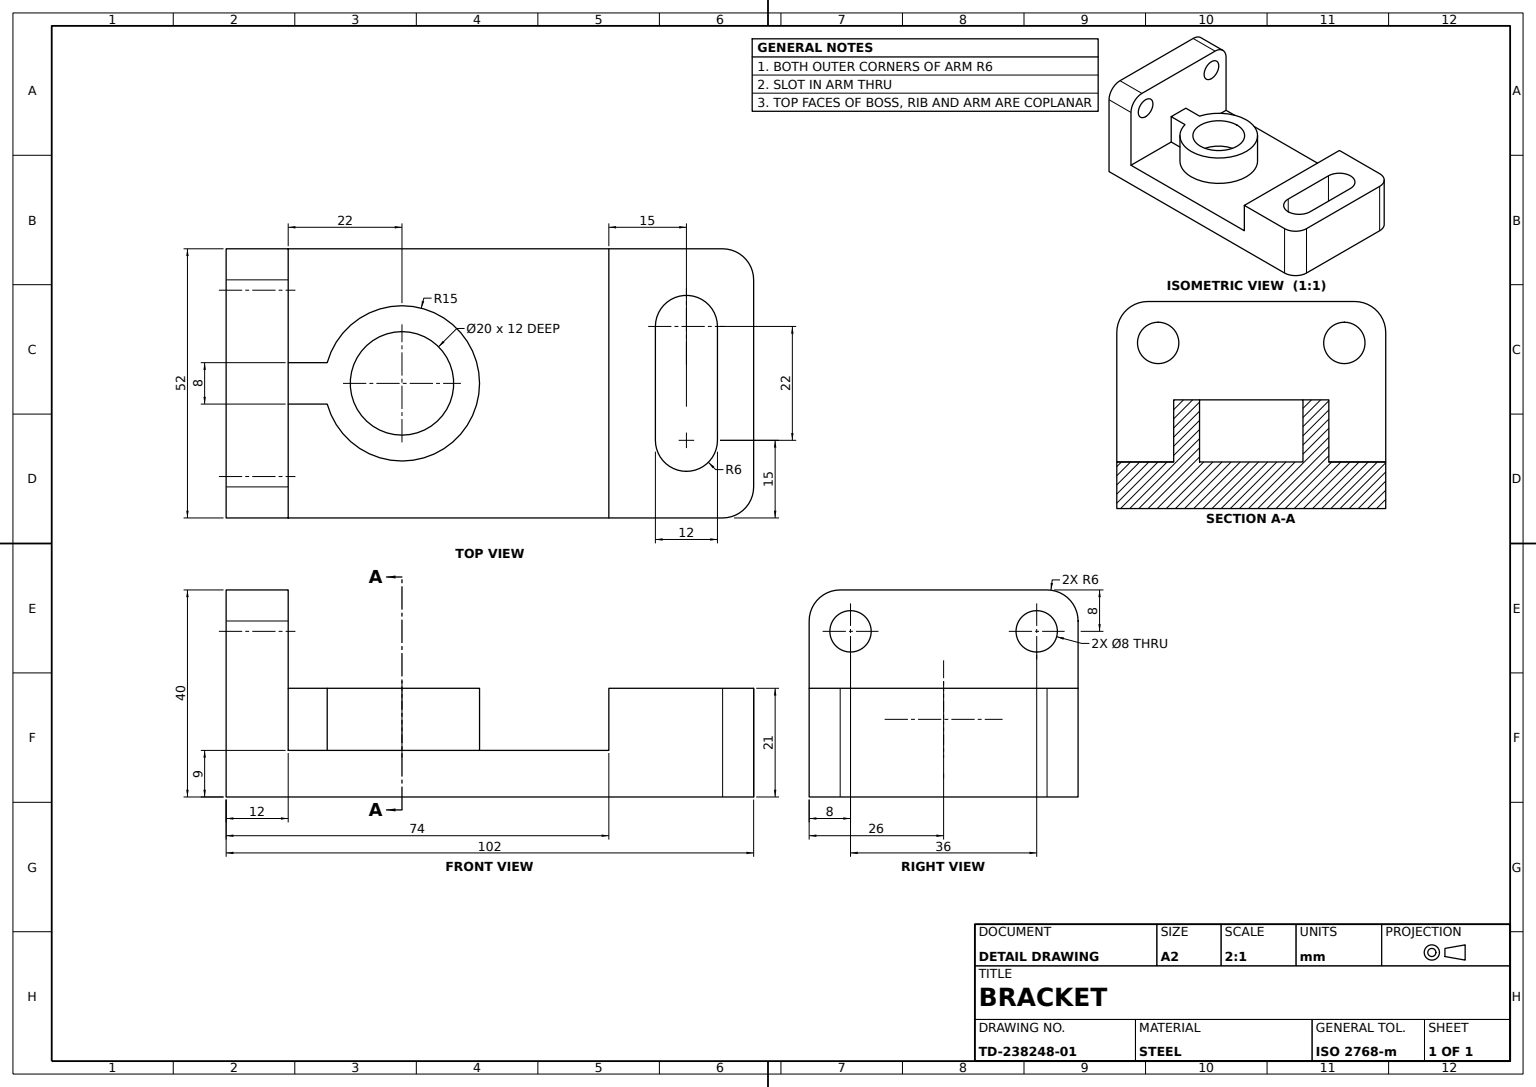
SolidWorks part; units mm, degrees
material "Plain Carbon Steel"
ref_plane "Front Plane" through (0, 0, 0) normal (0, 0, 1) x (1, 0, 0)
ref_plane "Top Plane" through (0, 0, 0) normal (0, 1, 0) x (1, 0, 0)
ref_plane "Right Plane" through (0, 0, 0) normal (1, 0, 0) x (0, 0, -1)
sketch "Back Plate Sketch" plane through (0, 0, 0) normal (0, 0, 1) x (1, 0, 0)
  line L0 (0, 0) -> (52, 0)
  line L1 (52, 0) -> (52, 96)
  line L2 (46, 102) -> (6, 102)
  line L3 (0, 96) -> (0, 0)
  arc A0 (6, 102) -> (0, 96) centre (6, 96) ccw
  arc A1 (52, 96) -> (46, 102) centre (46, 96) ccw
  dimension "D1" = 12
  dimension "D2" = 12
  dimension "D3" = 6
  dimension "D4" = 52
  dimension "D5" = 102
extrude "Back Plate" add sketch "Back Plate Sketch" along normal blind 9
sketch "Top Arm Sketch" plane through (0, 0, 9) normal (0, 0, 1) x (1, 0, 0)
  line L0 (52, 74) -> (52, 96)
  line L1 (0, 0) -> (52, 0) construction
  line L2 (26, 74) -> (52, 74)
  line L3 (52, 0) -> (52, 96) construction
  line L4 (52, 74) -> (0, 74)
  line L5 (0, 96) -> (0, 0) construction
  line L6 (0, 74) -> (0, 96)
  line L8 (52, 96) -> (52, 74)
  line L9 (6, 102) -> (46, 102)
  arc A0 (6, 102) -> (0, 96) centre (6, 96) ccw
  arc A1 (52, 96) -> (46, 102) centre (46, 96) ccw
  line M1 (0, 96) -> (0, 0)
  line M3 (52, 0) -> (52, 96)
  arc M4 (52, 96) -> (46, 102) centre (46, 96) ccw
  line M5 (46, 102) -> (6, 102)
  arc M6 (6, 102) -> (0, 96) centre (6, 96) ccw
  dimension "D1" = 12
  dimension "D2" = 12
  dimension "D3" = 74
extrude "Top Arm" add sketch "Top Arm Sketch" along normal blind 12 contours L4 L2 M3 M4 M5 M6 M1
sketch "Top Arm Slot Sketch" plane through (0, 0, 21) normal (0, 0, 1) x (1, 0, 0)
  line L0 (52, 74) -> (52, 96) construction
  line L1 (52, 74) -> (0, 74) construction
  line L3 (26, 95) -> (15, 95)
  line L5 (15, 83) -> (37, 83)
  line L7 (37, 95) -> (26, 95)
  arc A0 (37, 83) -> (37, 95) centre (37, 89) ccw
  arc A1 (15, 95) -> (15, 83) centre (15, 89) ccw
  dimension "D1" = 12
  dimension "D2" = 12
  dimension "D3" = 6
  dimension "D4" = 15
  dimension "D5" = 26
  dimension "D6" = 15
extrude "Top Arm Slot" cut sketch "Top Arm Slot Sketch" against normal blind 21
sketch "Base Foot Sketch" plane through (0, 0, 0) normal (0, -1, 0) x (1, 0, 0)
  line L0 (0, 9) -> (0, 34)
  line L1 (52, 9) -> (52, 34)
  line L2 (6, 40) -> (46, 40)
  line L4 (0, 0) -> (52, 0) construction
  line L7 (0, 0) -> (52, 0)
  line L8 (52, 0) -> (52, 9)
  line L9 (52, 9) -> (0, 9)
  line L10 (0, 9) -> (0, 0)
  line L11 (0, 0) -> (52, 0)
  line L12 (52, 0) -> (52, 9)
  line L14 (0, 9) -> (0, 0)
  arc A0 (6, 40) -> (0, 34) centre (6, 34) ccw
  arc A1 (52, 34) -> (46, 40) centre (46, 34) ccw
  dimension "D1" = 12
  dimension "D2" = 12
  dimension "D4" = 6
  dimension "D3" = 0
  dimension "D5" = 40
extrude "Base Foot" add sketch "Base Foot Sketch" against normal blind 12
sketch "Mounting Holes Sketch" plane through (0, 12, 0) normal (0, 1, 0) x (1, 0, 0)
  line L0 (0, -34) -> (0, -9) construction
  line L1 (52, -9) -> (52, -34) construction
  line L2 (46, -40) -> (6, -40) construction
  circle A0 centre (8, -32) radius 4
  circle A1 centre (44, -32) radius 4
  dimension "D1" = 8
  dimension "D3" = 8
  dimension "D7" = 8
  dimension "D2" = 8
  dimension "D4" = 8
  dimension "D5" = 8
  dimension "D6" = 8
extrude "Mounting Holes 2xØ8" cut sketch "Mounting Holes Sketch" against normal blind 12
sketch "Bearing Boss Sketch" plane through (0, 0, 9) normal (0, 0, 1) x (1, 0, 0)
  line L0 (0, 74) -> (0, 12) construction
  line L3 (30, 19) -> (30, 12)
  line L4 (0, 12) -> (52, 12) construction
  line L5 (30, 12) -> (22, 12)
  line L6 (46, 12) -> (6, 12) construction
  line L7 (22, 12) -> (22, 19.5432)
  line L9 (30, 19.5432) -> (30, 19)
  arc A0 (30, 19.5432) -> (22, 19.5432) centre (26, 34) ccw
  dimension "D1" = 30
  dimension "D2" = 15
  dimension "D3" = 22
  dimension "D4" = 26
  dimension "D5" = 7
  dimension "D6" = 7.5432
extrude "Bearing Boss Ø30" add sketch "Bearing Boss Sketch" along normal blind 12
sketch "Bore Sketch" plane through (0, 0, 21) normal (0, 0, 1) x (1, 0, 0)
  circle A0 centre (26, 34) radius 10
  dimension "D1" = 20
  dimension "D2" = 20
extrude "Bore Ø20" cut sketch "Bore Sketch" against normal blind 12
